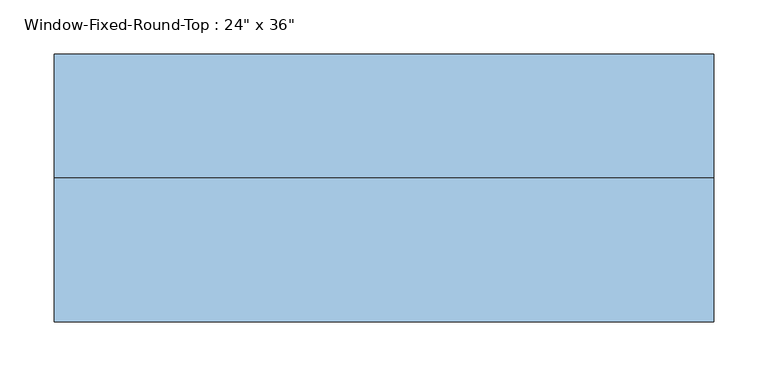
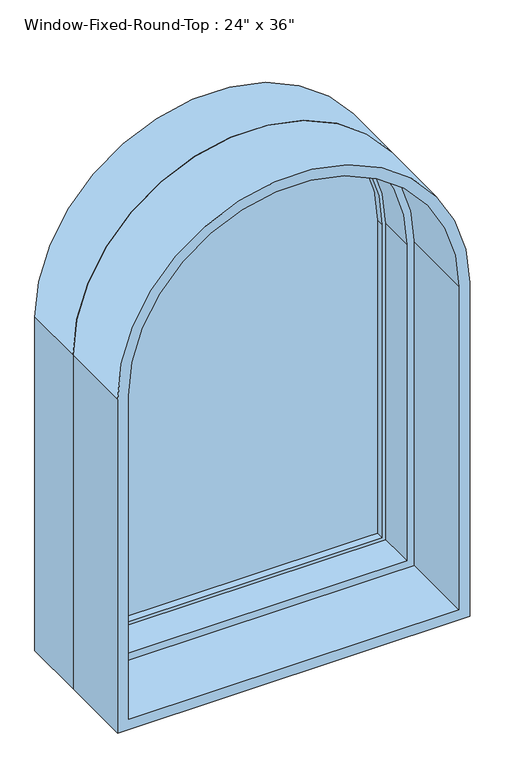
"""IFC4 building model written with IfcOpenShell, lengths in millimetres: window geometry."""

from ifc_helpers import new_model, si_unit, point, frame, frame_2d, origin, place, context, project, spatial, polyline, circle_curve, trimmed, segment, composite_curve, outline, extrude, source, transform, mapped, element, save
from ifc_brep_helpers import plane_surface, cylinder_surface, revolved_surface, advanced_brep


def window_2fd4accf(model_context):
    return source(origin(), model_context, "Body", "SolidModel", [
        advanced_brep(
        [(-273.05, 82.55, 1524.0), (-273.05, 19.05, 1524.0), (-273.05, 19.05, 946.15), (-273.05, 82.55, 946.15), (-292.1, 133.35, 1524.0), (-292.1, 82.55, 1524.0), (-292.1, 82.55, 927.1), (-292.1, 133.35, 927.1), (-304.8, 19.05, 1524.0), (-304.8, 133.35, 1524.0), (-304.8, 133.35, 914.4), (-304.8, 19.05, 914.4), (273.05, 19.05, 946.15), (273.05, 82.55, 946.15), (292.1, 82.55, 927.1), (292.1, 133.35, 927.1), (304.8, 133.35, 914.4), (304.8, 19.05, 914.4), (273.05, 19.05, 1524.0), (273.05, 82.55, 1524.0), (292.1, 82.55, 1524.0), (292.1, 133.35, 1524.0), (304.8, 133.35, 1524.0), (304.8, 19.05, 1524.0)],
        [
            (0, 1),
            (1, 2),
            (2, 3),
            (3, 0),
            (4, 5),
            (5, 6),
            (6, 7),
            (7, 4),
            (8, 9),
            (9, 10),
            (10, 11),
            (11, 8),
            (2, 12),
            (12, 13),
            (13, 3),
            (6, 14),
            (14, 15),
            (15, 7),
            (10, 16),
            (16, 17),
            (17, 11),
            (12, 18),
            (18, 19),
            (19, 13),
            (14, 20),
            (20, 21),
            (21, 15),
            (16, 22),
            (22, 23),
            (23, 17),
            (23, 8, circle_curve(frame((0.0, 19.05, 1524.0), z_axis=(0.0, -1.0, 0.0), x_axis=(1.0, 0.0, 0.0)), 304.8)),
            (1, 18, circle_curve(frame((0.0, 19.05, 1524.0), z_axis=(0.0, 1.0, 0.0), x_axis=(1.0, 0.0, 0.0)), 273.05)),
            (0, 19, circle_curve(frame((0.0, 82.55, 1524.0), z_axis=(0.0, 1.0, 0.0), x_axis=(1.0, 0.0, 0.0)), 273.05)),
            (5, 20, circle_curve(frame((0.0, 82.55, 1524.0), z_axis=(0.0, 1.0, 0.0), x_axis=(1.0, 0.0, 0.0)), 292.1)),
            (4, 21, circle_curve(frame((0.0, 133.35, 1524.0), z_axis=(0.0, 1.0, 0.0), x_axis=(1.0, 0.0, 0.0)), 292.1)),
            (9, 22, circle_curve(frame((0.0, 133.35, 1524.0), z_axis=(0.0, 1.0, 0.0), x_axis=(1.0, 0.0, 0.0)), 304.8)),
        ],
        [
            plane_surface(frame((-273.05, 19.05, 1524.0), z_axis=(1.0, 0.0, 0.0), x_axis=(0.0, 0.0, -1.0))),
            plane_surface(frame((-292.1, 82.55, 1524.0), z_axis=(1.0, 0.0, 0.0), x_axis=(0.0, 0.0, -1.0))),
            plane_surface(frame((-304.8, 133.35, 1524.0), z_axis=(-1.0, 0.0, 0.0), x_axis=(0.0, 0.0, -1.0))),
            plane_surface(frame((-273.05, 19.05, 946.15), z_axis=(0.0, 0.0, 1.0), x_axis=(1.0, 0.0, 0.0))),
            plane_surface(frame((-292.1, 82.55, 927.1), z_axis=(0.0, 0.0, 1.0), x_axis=(1.0, 0.0, 0.0))),
            plane_surface(frame((-304.8, 133.35, 914.4), z_axis=(0.0, 0.0, -1.0), x_axis=(1.0, 0.0, 0.0))),
            plane_surface(frame((273.05, 19.05, 946.15), z_axis=(-1.0, 0.0, 0.0), x_axis=(0.0, 0.0, 1.0))),
            plane_surface(frame((292.1, 82.55, 927.1), z_axis=(-1.0, 0.0, 0.0), x_axis=(0.0, 0.0, 1.0))),
            plane_surface(frame((304.8, 133.35, 914.4), z_axis=(1.0, 0.0, 0.0), x_axis=(0.0, 0.0, 1.0))),
            plane_surface(frame((0.0, 19.05, 1524.0), z_axis=(0.0, -1.0, 0.0), x_axis=(1.0, 0.0, 0.0))),
            revolved_surface(polyline([(273.05, 19.049999999999997, 1524.0), (273.05, 82.55, 1524.0)]), (0.0, 127.0, 1524.0), (0.0, -1.0, 0.0)),
            plane_surface(frame((0.0, 82.55, 1524.0), z_axis=(0.0, 1.0, 0.0), x_axis=(1.0, 0.0, 0.0))),
            revolved_surface(polyline([(292.1, 82.55, 1524.0), (292.1, 133.35, 1524.0)]), (0.0, 127.0, 1524.0), (0.0, -1.0, 0.0)),
            plane_surface(frame((0.0, 133.35, 1524.0), z_axis=(0.0, 1.0, 0.0), x_axis=(1.0, 0.0, 0.0))),
            cylinder_surface(frame((0.0, 127.0, 1524.0), z_axis=(0.0, -1.0, 0.0), x_axis=(1.0, 0.0, 0.0)), 304.8),
        ],
        [
            (0, [[1, 2, 3, 4]]),
            (1, [[5, 6, 7, 8]]),
            (2, [[9, 10, 11, 12]]),
            (3, [[-3, 13, 14, 15]]),
            (4, [[-7, 16, 17, 18]]),
            (5, [[-11, 19, 20, 21]]),
            (6, [[-14, 22, 23, 24]]),
            (7, [[-17, 25, 26, 27]]),
            (8, [[-20, 28, 29, 30]]),
            (9, [[-21, -30, 31, -12], [32, -22, -13, -2]]),
            (10, [[33, -23, -32, -1]]),
            (11, [[34, -25, -16, -6], [-15, -24, -33, -4]]),
            (12, [[35, -26, -34, -5]]),
            (13, [[36, -28, -19, -10], [-18, -27, -35, -8]]),
            (14, [[-31, -29, -36, -9]]),
        ],
    ),
        extrude(outline(composite_curve([segment(trimmed(circle_curve(frame_2d((1524.0, 0.0)), 304.8), [point((1524.0, 304.8))], [point((1524.0, -304.8))], False, "CARTESIAN"), True, "CONTINUOUS"), segment(polyline([(1524.0, -304.8), (914.4, -304.8), (914.4, 304.8), (1524.0, 304.8)]), True, "CONTINUOUS")], self_intersect=False), holes=[composite_curve([segment(polyline([(1524.0, 285.75), (933.45, 285.75), (933.45, -285.75), (1524.0, -285.75)]), True, "CONTINUOUS"), segment(trimmed(circle_curve(frame_2d((1524.0, 0.0)), 285.75), [point((1524.0, -285.75))], [point((1524.0, 285.75))], True, "CARTESIAN"), True, "CONTINUOUS")], self_intersect=False)]), frame((0.0, -114.3, 0.0), z_axis=(0.0, 1.0, 0.0), x_axis=(0.0, 0.0, 1.0)), (0.0, 0.0, 1.0), 133.35),
        extrude(outline(composite_curve([segment(polyline([(927.1, 292.1), (1524.0, 292.1)]), True, "CONTINUOUS"), segment(trimmed(circle_curve(frame_2d((1524.0, 0.0)), 292.1), [point((1524.0, 292.1))], [point((1524.0, -292.1))], False, "CARTESIAN"), True, "CONTINUOUS"), segment(polyline([(1524.0, -292.1), (927.1, -292.1), (927.1, 292.1)]), True, "CONTINUOUS")], self_intersect=False), holes=[composite_curve([segment(polyline([(952.5, -266.7), (1524.0, -266.7)]), True, "CONTINUOUS"), segment(trimmed(circle_curve(frame_2d((1524.0, 0.0)), 266.7), [point((1524.0, -266.7))], [point((1524.0, 266.7))], True, "CARTESIAN"), True, "CONTINUOUS"), segment(polyline([(1524.0, 266.7), (952.5, 266.7), (952.5, -266.7)]), True, "CONTINUOUS")], self_intersect=False)]), frame((0.0, 82.55, 0.0), z_axis=(0.0, 1.0, 0.0), x_axis=(0.0, 0.0, 1.0)), (0.0, 0.0, 1.0), 31.75),
        extrude(outline(composite_curve([segment(trimmed(circle_curve(frame_2d((1524.0, 0.0)), 266.7), [point((1524.0, 266.7))], [point((1524.0, -266.7))], False, "CARTESIAN"), True, "CONTINUOUS"), segment(polyline([(1524.0, -266.7), (952.5, -266.7), (952.5, 266.7), (1524.0, 266.7)]), True, "CONTINUOUS")], self_intersect=False)), frame((0.0, 107.95, 0.0), z_axis=(0.0, 1.0, 0.0), x_axis=(0.0, 0.0, 1.0)), (0.0, 0.0, 1.0), 6.35),
        extrude(outline(composite_curve([segment(trimmed(circle_curve(frame_2d((1524.0, 0.0)), 266.7), [point((1524.0, 266.7))], [point((1524.0, -266.7))], False, "CARTESIAN"), True, "CONTINUOUS"), segment(polyline([(1524.0, -266.7), (952.5, -266.7), (952.5, 266.7), (1524.0, 266.7)]), True, "CONTINUOUS")], self_intersect=False)), frame((0.0, 95.25, 0.0), z_axis=(0.0, 1.0, 0.0), x_axis=(0.0, 0.0, 1.0)), (0.0, 0.0, 1.0), 6.35),
        extrude(outline(composite_curve([segment(polyline([(1524.0, -292.1), (927.1, -292.1), (927.1, 292.1), (1524.0, 292.1)]), True, "CONTINUOUS"), segment(trimmed(circle_curve(frame_2d((1524.0, 0.0)), 292.1), [point((1524.0, 292.1))], [point((1524.0, -292.1))], False, "CARTESIAN"), True, "CONTINUOUS")], self_intersect=False), holes=[composite_curve([segment(polyline([(1524.0, 266.7), (952.5, 266.7), (952.5, -266.7), (1524.0, -266.7)]), True, "CONTINUOUS"), segment(trimmed(circle_curve(frame_2d((1524.0, 0.0)), 266.7), [point((1524.0, -266.7))], [point((1524.0, 266.7))], True, "CARTESIAN"), True, "CONTINUOUS")], self_intersect=False)]), frame((0.0, 114.3, 0.0), z_axis=(0.0, 1.0, 0.0), x_axis=(0.0, 0.0, 1.0)), (0.0, 0.0, 1.0), 12.7),
    ])


if __name__ == "__main__":
    model = new_model("IFC4")
    model_context = context("Model", 3, world=origin())
    ifc_project = project(units=[si_unit("LENGTHUNIT", "METRE", prefix="MILLI")], contexts=[model_context])
    site = spatial("IfcSite", under=ifc_project)
    building = spatial("IfcBuilding", under=site)
    placement = place(None, origin())
    window_shape = window_2fd4accf(model_context)
    element("IfcWindow", 1, ObjectType="Window-Fixed-Round-Top : 24\" x 36\"", at=placement, inside=building, context=model_context, shape_type="MappedRepresentation", body=[
        mapped(window_shape, transform((0.0, 0.0, 0.0), x_axis=(1.0, 0.0, 0.0), y_axis=(0.0, 1.0, 0.0), z_axis=(0.0, 0.0, 1.0))),
    ])
    save(model, "model.ifc")

# Revit data of these elements
# Type "Window-Fixed-Round-Top : 24\" x 36\""
#   Type Mark = "31"
#   Fire Rating = "0.5h"
#   Assembly Code = "B2020100"
#   Analytic Construction = "Double glazing - domestic"
#   Window Inset [instance default] = 0' - 0"
#   Wall Thickness [instance default] = 0' - 6"
#   Visual Light Transmittance = 0.81
#   Thermal Resistance (R) = 1.8146 (h·ft²·°F)/BTU
#   Solar Heat Gain Coefficient = 0.76
#   Rough Width = 2' - 0 1/2"
#   Rough Height = 3' - 0 1/2"
#   Interior Wall Closure [instance default] = 0' - 2 1/4"
#   Height = 3' - 0"
#   Heat Transfer Coefficient (U) = 0.5511 BTU/(h·ft²·°F)
#   Frame Extension [instance default] = 0' - 0 1/4"
#   Exterior Wall Closure [instance default] = 0' - 1 1/4"
#   Extension Jamb [instance default] = 0' - 2 1/4"
#   Default Sill Height = 3' - 0"
#   Width = 2' - 0"
#   Interior Trim Visibility [instance default] = yes
#   Exterior Trim Visibility [instance default] = yes
#   Extension Jamb Visibility [instance default] = yes
#   Interior Trim Material = Wood - Stained
#   Interior Trim = Trim-Window-Interior-Flat-Arch-Top-Tree_Centered : Picture Frame
#   Interior Frame Material = Wood - Stained
#   Glass Panel Material = Glass
#   Exterior Trim Material = Clad - White
#   Exterior Trim = Trim-Window-Exterior-Flat-Arch-Top-Tree_Centered : with Sill
#   Exterior Frame Material = Clad - White
#   Wall Closure = (empty or 0)
# Element 1 (IfcWindow, "Window-Fixed-Round-Top : 24\" x 36\"")
#   Wall Thickness = 0' - 9"
#   Extension Jamb = 0' - 5 1/4"
#   Materials on its faces: "Wood - Stained", "Clad - White", "Glass"
# Materials
#   "Wood - Stained": class "Wood", colour RGB 224 178 126, transparency 0, Cost = 0
#   "Glass": class "Glass", colour RGB 0 128 192, transparency 0.75, Description = "Soda Lime Glass", Cost = 0
#   "Clad - White": class "Wood", colour RGB 242 242 238, transparency 0, Cost = 0
